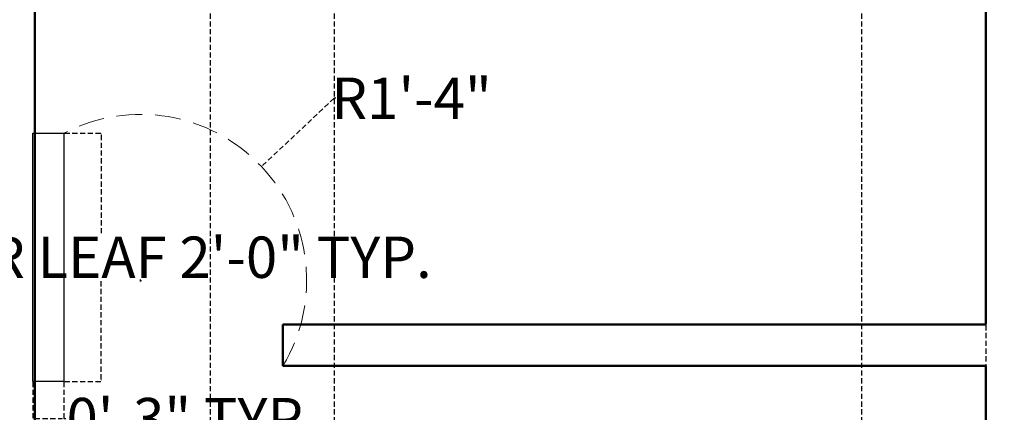
# Model space of a CAD drawing. Units: inches. Extents: x 513 to 1142, y 396 to 927.
# Tile 19 of 31: x 743 to 838, y 766 to 804. Entities that reach past the tile are written whole.
import ezdxf

# ---------------------------------------------------------------- set-up
doc = ezdxf.new("R2010")
doc.units = ezdxf.units.IN
doc.header["$MEASUREMENT"] = 0
doc.linetypes.add('DASHED', pattern=[0.75, 0.5, -0.25])
for name, color, linetype, lineweight in [('A-ANNO-DIMS', 2, 'DASHED', 18), ('A-DOOR', 4, 'Continuous', 25), ('A-DOOR-SWNG', 4, 'DASHED', 13), ('A-WALL', 7, 'Continuous', 50)]:
    doc.layers.add(name, color=color, linetype=linetype, lineweight=lineweight)
doc.styles.get("Standard").update_dxf_attribs({"font": 'arial.ttf'})
doc.dimstyles.get("Standard").update_dxf_attribs({"dimtxt": 4, "dimasz": 0.18, "dimexe": 0.18, "dimexo": 0.0625, "dimgap": 0.09, "dimtad": 0, "dimtih": 1, "dimtoh": 1, "dimdec": 0, "dimrnd": 6, "dimzin": 0, "dimdsep": 46, "dimlunit": 3, "dimtxsty": 'Standard', "dimcen": 0.09, "dimadec": 0, "dimazin": 0, "dimtfac": 1, "dimtdec": 0, "dimtofl": 0, "dimtmove": 0, "dimatfit": 3, "dimfxl": 1, "dimtolj": 1, "dimtzin": 0, "dimarcsym": 0})

# ---------------------------------------------------------------- blocks, each defined once
blk = doc.blocks.new('DOOR-LEAF-24IN')
blk.add_lwpolyline([(3, 24), (3, 0), (0, 0), (0, 24)], close=True)
blk = doc.blocks.new('*D123')
at = {"layer": 'A-ANNO-DIMS', "color": 0, "lineweight": -2, "transparency": 16777216}
for p, q in [((746.865, 792.67), (750.582, 792.67)), ((750.402, 792.49), (750.402, 782.83)), ((750.402, 768.85), (750.402, 778.51)), ((746.865, 768.67), (750.582, 768.67))]:
    blk.add_line(p, q, dxfattribs=at)
at = {"layer": 'A-ANNO-DIMS', "color": 0, "transparency": 16777216}
for points in [[(750.372, 792.49), (750.432, 792.49), (750.402, 792.67)], [(750.372, 768.85), (750.432, 768.85), (750.402, 768.67)]]:
    blk.add_solid(points, dxfattribs=at)
at = {"layer": 'Defpoints', "color": 0, "transparency": 16777216}
for p in [(746.802, 792.67), (750.402, 792.67), (746.802, 768.67)]:
    blk.add_point(p, dxfattribs=at)
at = {"layer": 'A-ANNO-DIMS', "color": 0, "transparency": 16777216, "insert": (750.402, 780.67), "char_height": 4, "attachment_point": 5}
blk.add_mtext('\\A1;INTERIOR LEAF 2\'-0" TYP.', dxfattribs=at)
blk = doc.blocks.new('*D124')
at = {"layer": 'A-ANNO-DIMS', "color": 0, "lineweight": -2, "transparency": 16777216}
for p, q in [((743.802, 768.607), (743.802, 764.89)), ((746.802, 768.607), (746.802, 764.89)), ((743.982, 765.07), (746.622, 765.07)), ((746.802, 765.07), (746.982, 765.07))]:
    blk.add_line(p, q, dxfattribs=at)
at = {"layer": 'A-ANNO-DIMS', "color": 0, "transparency": 16777216}
for points in [[(743.982, 765.1), (743.982, 765.04), (743.802, 765.07)], [(746.622, 765.1), (746.622, 765.04), (746.802, 765.07)]]:
    blk.add_solid(points, dxfattribs=at)
at = {"layer": 'Defpoints', "color": 0, "transparency": 16777216}
for p in [(743.802, 768.67), (746.802, 768.67), (746.802, 765.07)]:
    blk.add_point(p, dxfattribs=at)
at = {"layer": 'A-ANNO-DIMS', "color": 0, "transparency": 16777216, "insert": (759.263, 765.07), "char_height": 4, "attachment_point": 5}
blk.add_mtext('\\A1;0\'-3" TYP.', dxfattribs=at)
blk = doc.blocks.new('*D136')
at = {"layer": 'A-ANNO-DIMS', "color": 0, "lineweight": -2, "transparency": 16777216}
for p, q in [((835.995, 770.096), (835.995, 401.578)), ((743.802, 768.607), (743.802, 401.578)), ((743.982, 401.758), (784.509, 401.758)), ((835.815, 401.758), (795.289, 401.758))]:
    blk.add_line(p, q, dxfattribs=at)
at = {"layer": 'A-ANNO-DIMS', "color": 0, "transparency": 16777216}
for points in [[(743.982, 401.788), (743.982, 401.728), (743.802, 401.758)], [(835.815, 401.788), (835.815, 401.728), (835.995, 401.758)]]:
    blk.add_solid(points, dxfattribs=at)
at = {"layer": 'Defpoints', "color": 0, "transparency": 16777216}
for p in [(835.995, 770.158), (743.802, 768.67), (835.995, 401.758)]:
    blk.add_point(p, dxfattribs=at)
at = {"layer": 'A-ANNO-DIMS', "color": 0, "transparency": 16777216, "insert": (789.899, 401.758), "char_height": 4, "attachment_point": 5}
blk.add_mtext('\\A1;7\'-8"', dxfattribs=at)
blk = doc.blocks.new('*D167')
at = {"layer": 'A-ANNO-DIMS', "color": 0, "lineweight": -2, "transparency": 16777216}
for p, q in [((760.995, 637.221), (760.995, 920.738)), ((761.175, 920.558), (761.777, 920.558)), ((772.815, 920.558), (772.214, 920.558)), ((772.995, 637.221), (772.995, 920.738))]:
    blk.add_line(p, q, dxfattribs=at)
at = {"layer": 'A-ANNO-DIMS', "color": 0, "transparency": 16777216}
for points in [[(761.175, 920.588), (761.175, 920.528), (760.995, 920.558)], [(772.815, 920.588), (772.815, 920.528), (772.995, 920.558)]]:
    blk.add_solid(points, dxfattribs=at)
at = {"layer": 'Defpoints', "color": 0, "transparency": 16777216}
for p in [(772.995, 920.558), (760.995, 637.158), (772.995, 637.158)]:
    blk.add_point(p, dxfattribs=at)
at = {"layer": 'A-ANNO-DIMS', "color": 0, "transparency": 16777216, "insert": (766.995, 920.558), "char_height": 4, "attachment_point": 5}
blk.add_mtext('\\A1;1\'-0"', dxfattribs=at)
blk = doc.blocks.new('*D169')
at = {"layer": 'A-ANNO-DIMS', "color": 0, "lineweight": -2, "transparency": 16777216}
for p, q in [((835.995, 774.096), (835.995, 401.578)), ((839.995, 774.096), (839.995, 401.578)), ((836.175, 401.758), (839.815, 401.758)), ((839.995, 401.758), (840.175, 401.758))]:
    blk.add_line(p, q, dxfattribs=at)
at = {"layer": 'A-ANNO-DIMS', "color": 0, "transparency": 16777216}
for points in [[(836.175, 401.788), (836.175, 401.728), (835.995, 401.758)], [(839.815, 401.788), (839.815, 401.728), (839.995, 401.758)]]:
    blk.add_solid(points, dxfattribs=at)
at = {"layer": 'Defpoints', "color": 0, "transparency": 16777216}
for p in [(835.995, 774.158), (839.995, 774.158), (839.995, 401.758)]:
    blk.add_point(p, dxfattribs=at)
at = {"layer": 'A-ANNO-DIMS', "color": 0, "transparency": 16777216, "insert": (845.582, 401.758), "char_height": 4, "attachment_point": 5}
blk.add_mtext('\\A1;0\'-4"', dxfattribs=at)
blk = doc.blocks.new('*D175')
at = {"layer": 'A-ANNO-DIMS', "color": 0, "lineweight": -2, "transparency": 16777216}
for p, q in [((772.995, 637.221), (772.995, 920.738)), ((773.175, 920.558), (793.008, 920.558)), ((823.815, 920.558), (803.982, 920.558)), ((823.995, 637.221), (823.995, 920.738))]:
    blk.add_line(p, q, dxfattribs=at)
at = {"layer": 'A-ANNO-DIMS', "color": 0, "transparency": 16777216}
for points in [[(773.175, 920.588), (773.175, 920.528), (772.995, 920.558)], [(823.815, 920.588), (823.815, 920.528), (823.995, 920.558)]]:
    blk.add_solid(points, dxfattribs=at)
at = {"layer": 'Defpoints', "color": 0, "transparency": 16777216}
for p in [(823.995, 920.558), (772.995, 637.158), (823.995, 637.158)]:
    blk.add_point(p, dxfattribs=at)
at = {"layer": 'A-ANNO-DIMS', "color": 0, "transparency": 16777216, "insert": (798.495, 920.558), "char_height": 4, "attachment_point": 5}
blk.add_mtext('\\A1;4\'-3"', dxfattribs=at)
blk = doc.blocks.new('*D191')
at = {"layer": 'A-ANNO-DIMS', "color": 0, "lineweight": -2, "transparency": 16777216}
for p, q in [((772.934, 796.041), (766.048, 789.558)), ((773.114, 796.041), (772.934, 796.041)), ((754.132, 778.423), (754.312, 778.423)), ((754.222, 778.333), (754.222, 778.513))]:
    blk.add_line(p, q, dxfattribs=at)
at = {"layer": 'A-ANNO-DIMS', "color": 0, "transparency": 16777216}
blk.add_solid([(766.028, 789.579), (766.069, 789.536), (765.917, 789.434)], dxfattribs=at)
at = {"layer": 'Defpoints', "color": 0, "transparency": 16777216}
for p in [(765.917, 789.434), (754.222, 778.423)]:
    blk.add_point(p, dxfattribs=at)
at = {"layer": 'A-ANNO-DIMS', "color": 0, "transparency": 16777216, "insert": (780.435, 796.041), "char_height": 4, "attachment_point": 5}
blk.add_mtext('\\A1;R1\'-4"', dxfattribs=at)

msp = doc.modelspace()

# ---------------------------------------------------------------- linework, layer by layer
at = {"layer": 'A-DOOR-SWNG', "ltscale": 5}
msp.add_arc((754.222, 778.423), 16.063, 329.03262, 117.51161, dxfattribs=at)
at = {"layer": 'A-WALL'}
for p, q in [((743.995, 870.158), (743.995, 710.158)), ((835.995, 870.158), (835.995, 774.158)), ((767.995, 774.158), (767.995, 770.158)), ((835.995, 774.158), (767.995, 774.158)), ((835.995, 770.158), (767.995, 770.158)), ((835.995, 770.158), (835.995, 641.158))]:
    msp.add_line(p, q, dxfattribs=at)

# ---------------------------------------------------------------- block references
at = {"layer": 'A-DOOR'}
msp.add_blockref('DOOR-LEAF-24IN', (743.802, 768.67), dxfattribs=at)

# ---------------------------------------------------------------- dimensions: what is measured, and where the dimension line sits
at = {"layer": 'A-ANNO-DIMS'}
for base, p1, p2, picture, middle in [((772.995, 920.558), (760.995, 637.158), (772.995, 637.158), '*D167', (766.995, 920.558)), ((823.995, 920.558), (772.995, 637.158), (823.995, 637.158), '*D175', (798.495, 920.558)), ((839.995, 401.758), (835.995, 774.158), (839.995, 774.158), '*D169', (845.582, 401.758)), ((835.995, 401.758), (743.802, 768.67), (835.995, 770.158), '*D136', (789.899, 401.758))]:
    dim = msp.add_linear_dim(base=base, p1=p1, p2=p2, dimstyle='Standard', override={"dimdec": 1, "dimlfac": 1, "dimrnd": 0, "dimzin": 1, "dimdsep": 46, "dimlunit": 4, "dimfrac": 2}, dxfattribs=at)
    dim.commit()
    dim.dimension.update_dxf_attribs({"geometry": picture, "text_midpoint": middle})
dim = msp.add_radius_dim(center=(754.222, 778.423), mpoint=(765.917, 789.434), dimstyle='Standard', override={"dimdec": 1, "dimlfac": 1, "dimrnd": 0, "dimzin": 1, "dimdsep": 46, "dimlunit": 4, "dimfrac": 2}, dxfattribs=at)
dim.commit()
dim.dimension.update_dxf_attribs({"geometry": '*D191', "text_midpoint": (780.435, 796.041), "dimtype": 164})
dim = msp.add_linear_dim(base=(750.402, 792.67), p1=(746.802, 768.67), p2=(746.802, 792.67), angle=90, text='INTERIOR LEAF <> TYP.', dimstyle='Standard', override={"dimdec": 1, "dimlfac": 1, "dimrnd": 0, "dimzin": 1, "dimdsep": 46, "dimlunit": 4, "dimfrac": 2}, dxfattribs=at)
dim.commit()
dim.dimension.update_dxf_attribs({"geometry": '*D123', "text_midpoint": (750.402, 780.67)})
dim = msp.add_linear_dim(base=(746.802, 765.07), p1=(743.802, 768.67), p2=(746.802, 768.67), text='<> TYP.', dimstyle='Standard', override={"dimdec": 1, "dimlfac": 1, "dimrnd": 0, "dimzin": 1, "dimdsep": 46, "dimlunit": 4, "dimfrac": 2}, dxfattribs=at)
dim.commit()
dim.dimension.update_dxf_attribs({"geometry": '*D124', "text_midpoint": (759.263, 765.07)})

doc.saveas('drawing.dxf')
